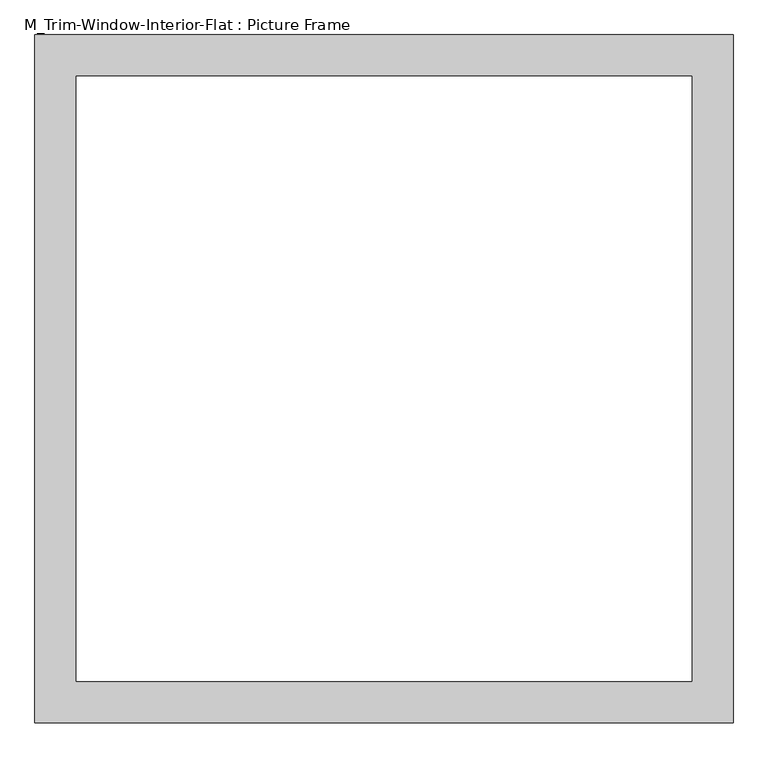
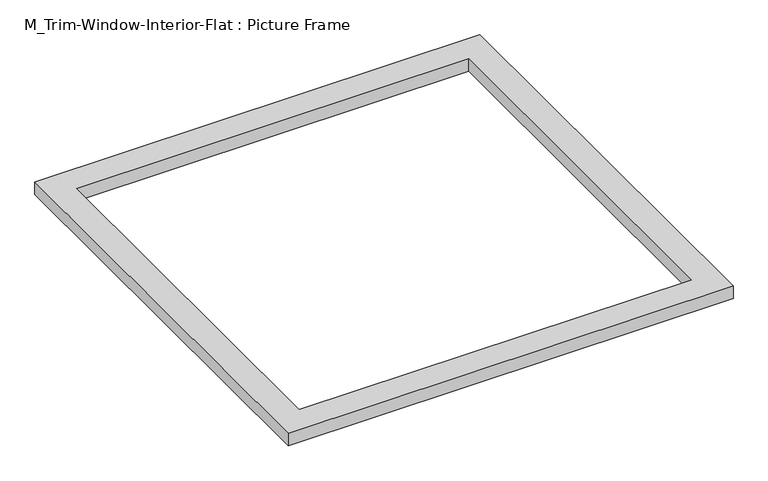
"""IFC4 building model written with IfcOpenShell, lengths in millimetres: proxy geometry, M_Trim-Window-Interior-Flat : Picture Frame."""

from ifc_helpers import new_model, si_unit, origin, origin_with_axes, place, context, project, spatial, polyline, outline, extrude, source, transform, mapped, element, save


def m_trim_window_interior_flat_picture_frame_b6dd03a6(model_context):
    return source(origin(), model_context, "Body", "SweptSolid", [
        extrude(outline(polyline([(504.5, 47.3), (504.5, -947.3), (-504.5, -947.3), (-504.5, 47.3), (504.5, 47.3)]), holes=[polyline([(444.5, -12.7), (-444.5, -12.7), (-444.5, -887.3), (444.5, -887.3), (444.5, -12.7)])]), origin_with_axes(), (0.0, 0.0, 1.0), 30.0),
    ])


if __name__ == "__main__":
    model = new_model("IFC4")
    model_context = context("Model", 3, world=origin())
    ifc_project = project(units=[si_unit("LENGTHUNIT", "METRE", prefix="MILLI")], contexts=[model_context])
    site = spatial("IfcSite", under=ifc_project)
    building = spatial("IfcBuilding", under=site)
    placement = place(None, origin())
    m_trim_window_interior_flat_picture_frame_shape = m_trim_window_interior_flat_picture_frame_b6dd03a6(model_context)
    element("IfcBuildingElementProxy", 1, Name="M_Trim-Window-Interior-Flat : Picture Frame", ObjectType="M_Trim-Window-Interior-Flat : Picture Frame", at=placement, inside=building, context=model_context, shape_type="MappedRepresentation", body=[
        mapped(m_trim_window_interior_flat_picture_frame_shape, transform((0.0, 0.0, 0.0), x_axis=(1.0, 0.0, 0.0), y_axis=(0.0, 1.0, 0.0), z_axis=(0.0, 0.0, 1.0))),
    ])
    save(model, "model.ifc")

# Revit data of these elements
# Type "M_Trim-Window-Interior-Flat : Picture Frame"
#   Trim Thickness_Picture Frame = 0' - 1.1811"
#   Trim Width = 0' - 2.3622"
#   Trim Thickness_with Sill = 0' - 0.7874"
#   Sill Thickness = 0' - 1.1811"
#   Opening Width [instance default] = 1' - 11.62205"
#   Opening Height [instance default] = 2' - 11.43307"
#   Default Elevation = 3' - 11.24409"
#   Sill = no
#   Picture Frame = yes
#   Trim Material [instance default] = none
# Element 1 (IfcBuildingElementProxy, "M_Trim-Window-Interior-Flat : Picture Frame")
#   Opening Width = 3' - 0"
#   Trim Material = Wood - Stained
#   Materials on its faces: "Wood - Stained"
# Materials
#   "Wood - Stained": class "Wood", colour RGB 227 170 128, transparency 0, Cost = 0
